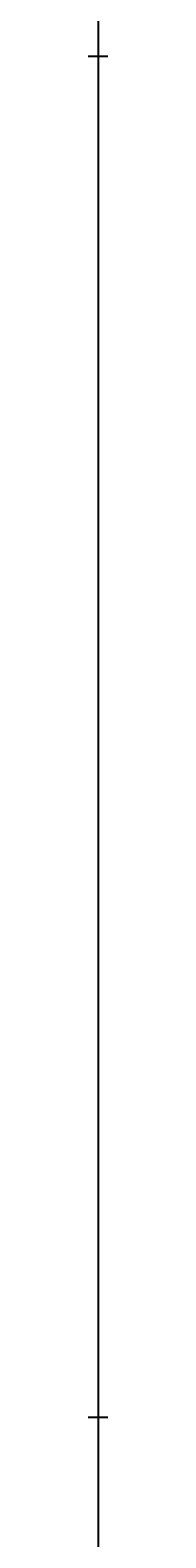
# Model space of a CAD drawing. Units: inches. Extents: x 35362 to 73946, y 43607 to 67532.
# Tile 28 of 134: x 48373 to 48373, y 46091 to 46564. Entities that reach past the tile are written whole.
import ezdxf

# ---------------------------------------------------------------- set-up
doc = ezdxf.new("R2010")
doc.units = ezdxf.units.IN
doc.header["$MEASUREMENT"] = 0
doc.layers.add('A-ANNO-DIMS', color=2, linetype='Continuous', lineweight=18)
doc.styles.get("Standard").update_dxf_attribs({"font": 'arial.ttf'})
doc.dimstyles.get("Standard").update_dxf_attribs({"dimtxt": 0.18, "dimasz": 0.18, "dimexe": 0.18, "dimexo": 0.0625, "dimgap": 0.09, "dimtad": 0, "dimtih": 1, "dimtoh": 1, "dimdec": 4, "dimzin": 0, "dimdsep": 46, "dimtxsty": 'Standard', "dimcen": 0.09, "dimadec": 0, "dimazin": 0, "dimtfac": 1, "dimtdec": 4, "dimtofl": 0, "dimtmove": 0, "dimatfit": 3, "dimfxl": 1, "dimtolj": 1, "dimtzin": 0, "dimarcsym": 0})

# ---------------------------------------------------------------- blocks, each defined once
blk = doc.blocks.new('*D5')
at = {"layer": 'A-ANNO-DIMS', "color": 0, "lineweight": -2, "transparency": 16777216}
for p, q in [((37121.95, 46919.32), (37121.95, 43606.68)), ((69871.5, 45449.83), (69871.5, 43606.68)), ((37122.13, 43606.86), (53496.29, 43606.86)), ((69871.32, 43606.86), (53497.15, 43606.86))]:
    blk.add_line(p, q, dxfattribs=at)
at = {"layer": 'A-ANNO-DIMS', "color": 0, "transparency": 16777216}
for points in [[(37122.13, 43606.89), (37122.13, 43606.83), (37121.95, 43606.86)], [(69871.32, 43606.89), (69871.32, 43606.83), (69871.5, 43606.86)]]:
    blk.add_solid(points, dxfattribs=at)
at = {"layer": 'Defpoints', "color": 0, "transparency": 16777216}
for p in [(37121.95, 46919.38), (69871.5, 45449.89), (69871.5, 43606.86)]:
    blk.add_point(p, dxfattribs=at)
at = {"layer": 'A-ANNO-DIMS', "color": 0, "transparency": 16777216, "insert": (53496.72, 43606.86), "char_height": 0.18, "attachment_point": 5}
blk.add_mtext('\\A1;32750', dxfattribs=at)
blk = doc.blocks.new('*D11')
at = {"layer": 'A-ANNO-DIMS', "color": 0, "lineweight": -2, "transparency": 16777216}
for p, q in [((47978.66, 56028.77), (47978.66, 43606.68)), ((53109.76, 56028.77), (53109.76, 43606.68)), ((47978.84, 43606.86), (50543.87, 43606.86)), ((53109.58, 43606.86), (50544.55, 43606.86))]:
    blk.add_line(p, q, dxfattribs=at)
at = {"layer": 'A-ANNO-DIMS', "color": 0, "transparency": 16777216}
for points in [[(47978.84, 43606.89), (47978.84, 43606.83), (47978.66, 43606.86)], [(53109.58, 43606.89), (53109.58, 43606.83), (53109.76, 43606.86)]]:
    blk.add_solid(points, dxfattribs=at)
at = {"layer": 'Defpoints', "color": 0, "transparency": 16777216}
for p in [(47978.66, 56028.84), (53109.76, 56028.84), (53109.76, 43606.86)]:
    blk.add_point(p, dxfattribs=at)
at = {"layer": 'A-ANNO-DIMS', "color": 0, "transparency": 16777216, "insert": (50544.21, 43606.86), "char_height": 0.18, "attachment_point": 5}
blk.add_mtext('\\A1;5131', dxfattribs=at)
blk = doc.blocks.new('*D27')
at = {"layer": 'A-ANNO-DIMS', "color": 0, "lineweight": -2, "transparency": 16777216}
for p, q in [((47978.66, 56028.77), (47978.66, 43606.68)), ((48373.49, 53428.96), (48373.49, 43606.68)), ((47978.84, 43606.86), (48175.68, 43606.86)), ((48373.31, 43606.86), (48176.47, 43606.86))]:
    blk.add_line(p, q, dxfattribs=at)
at = {"layer": 'A-ANNO-DIMS', "color": 0, "transparency": 16777216}
for points in [[(47978.84, 43606.89), (47978.84, 43606.83), (47978.66, 43606.86)], [(48373.31, 43606.89), (48373.31, 43606.83), (48373.49, 43606.86)]]:
    blk.add_solid(points, dxfattribs=at)
at = {"layer": 'Defpoints', "color": 0, "transparency": 16777216}
for p in [(47978.66, 56028.84), (48373.49, 53429.02), (48373.49, 43606.86)]:
    blk.add_point(p, dxfattribs=at)
at = {"layer": 'A-ANNO-DIMS', "color": 0, "transparency": 16777216, "insert": (48176.08, 43606.86), "char_height": 0.18, "attachment_point": 5}
blk.add_mtext('\\A1;394.8', dxfattribs=at)
blk = doc.blocks.new('*D67')
at = {"layer": 'A-ANNO-DIMS', "color": 0, "lineweight": -2, "transparency": 16777216}
for p, q in [((56873.54, 53351.53), (35361.77, 53351.53)), ((35361.95, 53351.35), (35361.95, 49400.89)), ((35361.95, 45450.07), (35361.95, 49400.53)), ((53793.58, 45449.89), (35361.77, 45449.89))]:
    blk.add_line(p, q, dxfattribs=at)
at = {"layer": 'A-ANNO-DIMS', "color": 0, "transparency": 16777216}
for points in [[(35361.92, 53351.35), (35361.98, 53351.35), (35361.95, 53351.53)], [(35361.92, 45450.07), (35361.98, 45450.07), (35361.95, 45449.89)]]:
    blk.add_solid(points, dxfattribs=at)
at = {"layer": 'Defpoints', "color": 0, "transparency": 16777216}
for p in [(35361.95, 53351.53), (56873.6, 53351.53), (53793.64, 45449.89)]:
    blk.add_point(p, dxfattribs=at)
at = {"layer": 'A-ANNO-DIMS', "color": 0, "transparency": 16777216, "insert": (35361.95, 49400.71), "char_height": 0.18, "attachment_point": 5}
blk.add_mtext('\\A1;7901.6', dxfattribs=at)
blk = doc.blocks.new('*D76')
at = {"layer": 'A-ANNO-DIMS', "color": 0, "lineweight": -2, "transparency": 16777216}
for p, q in [((54052.84, 46555.29), (35361.77, 46555.29)), ((35361.95, 46555.11), (35361.95, 46342.27)), ((35361.95, 46129.06), (35361.95, 46341.9)), ((53793.58, 46128.88), (35361.77, 46128.88))]:
    blk.add_line(p, q, dxfattribs=at)
at = {"layer": 'A-ANNO-DIMS', "color": 0, "transparency": 16777216}
for points in [[(35361.92, 46555.11), (35361.98, 46555.11), (35361.95, 46555.29)], [(35361.92, 46129.06), (35361.98, 46129.06), (35361.95, 46128.88)]]:
    blk.add_solid(points, dxfattribs=at)
at = {"layer": 'Defpoints', "color": 0, "transparency": 16777216}
for p in [(35361.95, 46555.29), (54052.9, 46555.29), (53793.64, 46128.88)]:
    blk.add_point(p, dxfattribs=at)
at = {"layer": 'A-ANNO-DIMS', "color": 0, "transparency": 16777216, "insert": (35361.95, 46342.09), "char_height": 0.18, "attachment_point": 5}
blk.add_mtext('\\A1;426.4', dxfattribs=at)
blk = doc.blocks.new('*D90')
at = {"layer": 'A-ANNO-DIMS', "color": 0, "lineweight": -2, "transparency": 16777216}
for p, q in [((53707.72, 47291.29), (35361.77, 47291.29)), ((35361.95, 47291.11), (35361.95, 46710.26)), ((35361.95, 46129.06), (35361.95, 46709.9)), ((53793.58, 46128.88), (35361.77, 46128.88))]:
    blk.add_line(p, q, dxfattribs=at)
at = {"layer": 'A-ANNO-DIMS', "color": 0, "transparency": 16777216}
for points in [[(35361.92, 47291.11), (35361.98, 47291.11), (35361.95, 47291.29)], [(35361.92, 46129.06), (35361.98, 46129.06), (35361.95, 46128.88)]]:
    blk.add_solid(points, dxfattribs=at)
at = {"layer": 'Defpoints', "color": 0, "transparency": 16777216}
for p in [(53707.78, 47291.29), (35361.95, 46128.88), (53793.64, 46128.88)]:
    blk.add_point(p, dxfattribs=at)
at = {"layer": 'A-ANNO-DIMS', "color": 0, "transparency": 16777216, "insert": (35361.95, 46710.08), "char_height": 0.18, "attachment_point": 5}
blk.add_mtext('\\A1;1162.4', dxfattribs=at)

msp = doc.modelspace()

# ---------------------------------------------------------------- dimensions: what is measured, and where the dimension line sits
at = {"layer": 'A-ANNO-DIMS'}
for base, p1, p2, override, picture, middle in [((53109.76, 43606.859), (47978.665, 56028.836), (53109.76, 56028.836), {"dimdec": 0, "dimlfac": 1, "dimrnd": 0, "dimzin": 0, "dimdsep": 46, "dimlunit": 2}, '*D11', (50544.212, 43606.859)), ((48373.492, 43606.859), (47978.665, 56028.836), (48373.492, 53429.019), {"dimdec": 1, "dimlfac": 1, "dimrnd": 0, "dimzin": 0, "dimdsep": 46, "dimlunit": 2}, '*D27', (48176.078, 43606.859)), ((69871.496, 43606.859), (37121.949, 46919.381), (69871.496, 45449.894), {"dimdec": 0, "dimlfac": 1, "dimrnd": 0, "dimzin": 0, "dimdsep": 46, "dimlunit": 2}, '*D5', (53496.723, 43606.859))]:
    dim = msp.add_linear_dim(base=base, p1=p1, p2=p2, dimstyle='Standard', override=override, dxfattribs=at)
    dim.commit()
    dim.dimension.update_dxf_attribs({"geometry": picture, "text_midpoint": middle})
for base, p1, p2, picture, middle in [((35361.949, 53351.529), (53793.638, 45449.894), (56873.602, 53351.529), '*D67', (35361.949, 49400.712)), ((35361.949, 46128.878), (53707.781, 47291.285), (53793.638, 46128.878), '*D90', (35361.949, 46710.081)), ((35361.949, 46555.293), (53793.638, 46128.878), (54052.899, 46555.293), '*D76', (35361.949, 46342.086))]:
    dim = msp.add_linear_dim(base=base, p1=p1, p2=p2, angle=90, dimstyle='Standard', override={"dimdec": 1, "dimlfac": 1, "dimrnd": 0, "dimzin": 0, "dimdsep": 46, "dimlunit": 2}, dxfattribs=at)
    dim.commit()
    dim.dimension.update_dxf_attribs({"geometry": picture, "text_midpoint": middle})

doc.saveas('drawing.dxf')
